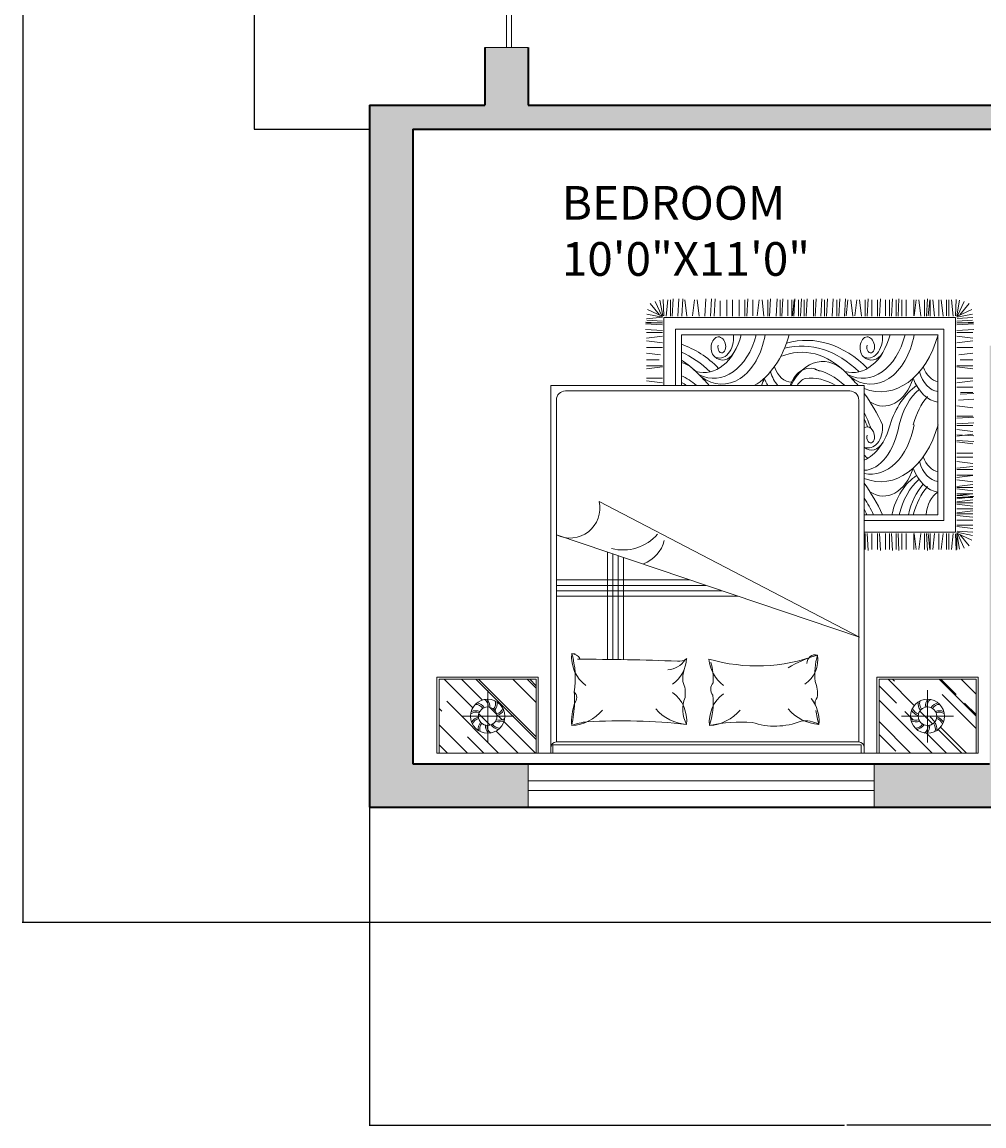
# Model space of a CAD drawing. Units: inches. Extents: x 2540 to 3167, y 3083 to 4007.
# Tile 1 of 15: x 2540 to 2740, y 3083 to 3313. Entities that reach past the tile are written whole.
import ezdxf

# ---------------------------------------------------------------- set-up
doc = ezdxf.new("R2010")
doc.units = ezdxf.units.IN
for name, color, linetype, lineweight in [('A-ANNO-DIMS', 2, 'Continuous', 18), ('A-AREA-IDEN', 7, 'Continuous', 18), ('A-DOOR', 4, 'Continuous', 18), ('A-FLOR-EDGE', 7, 'Continuous', 25), ('A-FURN', 8, 'Continuous', 13), ('A-GLAZ', 4, 'Continuous', 18)]:
    doc.layers.add(name, color=color, linetype=linetype, lineweight=lineweight)
doc.layers.add('A-WALL', color=143, linetype='Continuous', lineweight=35, true_color=0x7aafdf)
doc.layers.add('A-WALL-PATT', color=143, linetype='Continuous', lineweight=13, true_color=0x7aafdf)
doc.styles.get("Standard").update_dxf_attribs({"font": 'arial.ttf'})
doc.dimstyles.get("Standard").update_dxf_attribs({"dimtxt": 0.18, "dimasz": 0.18, "dimexe": 0.18, "dimexo": 0.0625, "dimgap": 0.09, "dimtad": 0, "dimtih": 1, "dimtoh": 1, "dimdec": 4, "dimzin": 0, "dimdsep": 46, "dimtxsty": 'Standard', "dimcen": 0.09, "dimadec": 0, "dimazin": 0, "dimtfac": 1, "dimtdec": 4, "dimtofl": 0, "dimtmove": 0, "dimatfit": 3, "dimfxl": 1, "dimtolj": 1, "dimtzin": 0, "dimarcsym": 0})

# ---------------------------------------------------------------- blocks, each defined once
blk = doc.blocks.new('A$C64B41DC1')
for p, q in [((0, 2.5079), (2.9903, 2.5079)), ((0, 2.0879), (0, 2.5079)), ((0.012, 2.4618), (0.0581, 2.5079)), ((0.012, 2.3515), (0.1684, 2.5079)), ((0.012, 2.0999), (0.012, 2.5079)), ((0.0543, 2.2213), (0.3409, 2.5079)), ((0.1689, 2.4179), (0.2589, 2.5079)), ((0.3265, 2.386), (0.4484, 2.5079)), ((0.3699, 2.3332), (0.5445, 2.5079)), ((0.548, 2.5079), (0.548, 2.0999)), ((0.56, 2.5079), (0.56, 2.0879)), ((0.6301, 2.5079), (0.6301, 0.4779)), ((0.6401, 2.461), (0.6401, 2.5079)), ((0.6401, 2.5079), (2.344, 2.5079)), ((2.344, 2.5079), (2.3601, 2.5079)), ((2.344, 2.5079), (2.344, 2.461)), ((2.3601, 2.5079), (2.3601, 2.4761)), ((2.3601, 0.4779), (2.3601, 2.5079)), ((2.4303, 2.5079), (2.4303, 2.0879)), ((2.4423, 2.5079), (2.4423, 2.0999)), ((2.4423, 2.3333), (2.6169, 2.5079)), ((2.4423, 2.2145), (2.7357, 2.5079)), ((2.705, 2.398), (2.8149, 2.5079)), ((2.7691, 2.3772), (2.8998, 2.5079)), ((2.7819, 2.3646), (2.9252, 2.5079)), ((2.9783, 2.0999), (2.9783, 2.5079)), ((2.9903, 2.0879), (2.9903, 2.5079)), ((0.2804, 2.1597), (0.2804, 2.4481)), ((2.344, 2.461), (0.6401, 2.461)), ((0.6601, 2.4461), (1.4951, 2.4461)), ((0.6601, 2.4461), (0.6601, 0.5579)), ((1.4951, 2.4461), (0.6697, 2.4461)), ((2.3301, 2.4461), (1.4951, 2.4461)), ((2.3301, 0.5579), (2.3301, 2.4461)), ((2.4423, 2.404), (2.5354, 2.4971)), ((2.7099, 2.1597), (2.7099, 2.4481)), ((0.2157, 2.0999), (0.548, 2.4322)), ((0.2299, 2.0999), (0.548, 2.418)), ((0.2311, 2.2906), (0.2937, 2.3532)), ((0.3405, 2.3039), (0.3605, 2.3238)), ((2.6158, 2.3088), (2.6313, 2.3243)), ((2.6674, 2.2756), (2.7382, 2.3464)), ((2.7249, 2.3076), (2.7512, 2.3339)), ((2.7914, 2.1846), (2.9783, 2.3715)), ((0.012, 2.261), (0.0275, 2.2765)), ((0.0404, 2.0999), (0.1982, 2.2578)), ((0.1362, 2.3039), (0.4246, 2.3039)), ((0.2905, 2.2539), (0.3304, 2.2938)), ((2.8541, 2.3039), (2.5657, 2.3039)), ((2.5849, 2.2779), (2.6158, 2.3088)), ((2.7746, 2.0999), (2.9783, 2.3036)), ((2.9144, 2.2312), (2.9783, 2.2951)), ((0.1365, 2.0999), (0.251, 2.2144)), ((0.4194, 2.0999), (0.548, 2.2285)), ((2.4423, 2.1353), (2.5382, 2.2312)), ((2.4918, 2.0999), (2.6366, 2.2447)), ((0.4986, 2.0999), (0.548, 2.1493)), ((0.5127, 2.0999), (0.548, 2.1352)), ((2.7831, 2.0999), (2.8678, 2.1846)), ((2.8962, 2.0999), (2.9783, 2.182)), ((0.56, 2.0879), (0, 2.0879)), ((0.548, 2.0999), (0.012, 2.0999)), ((2.4303, 2.0879), (2.9903, 2.0879)), ((2.4423, 2.0999), (2.9783, 2.0999)), ((2.5172, 2.0999), (2.5269, 2.1096)), ((0.9415, 1.9902), (0.9415, 1.3975)), ((0.9715, 1.9906), (0.9715, 1.4076)), ((1.0015, 1.991), (1.0015, 1.4177)), ((1.0315, 1.9916), (1.0315, 1.4279)), ((2.3349, 1.8678), (0.6613, 1.3029)), ((0.8956, 1.1191), (2.3349, 1.8678)), ((1.6636, 1.6412), (0.6601, 1.6412)), ((1.5748, 1.6112), (0.6601, 1.6112)), ((2.3665, 1.295), (2.3665, 1.3839)), ((2.377, 1.295), (2.3822, 1.3891)), ((2.4032, 1.295), (2.4032, 1.3839)), ((2.4346, 1.295), (2.4346, 1.3839)), ((2.4451, 1.295), (2.4503, 1.3891)), ((2.4774, 1.2957), (2.4774, 1.3837)), ((2.5, 1.295), (2.5, 1.3839)), ((2.5105, 1.295), (2.5157, 1.3891)), ((2.5367, 1.295), (2.5367, 1.3839)), ((2.5471, 1.295), (2.5524, 1.3891)), ((2.5681, 1.295), (2.5681, 1.3839)), ((2.5918, 1.295), (2.5918, 1.3839)), ((2.6346, 1.2957), (2.6346, 1.3837)), ((2.6362, 1.2957), (2.6467, 1.3839)), ((2.6729, 1.295), (2.6624, 1.3839)), ((2.6938, 1.295), (2.6938, 1.3839)), ((2.7043, 1.295), (2.7095, 1.3891)), ((2.7127, 1.2957), (2.7232, 1.3839)), ((2.7253, 1.295), (2.7253, 1.3839)), ((2.7494, 1.295), (2.7389, 1.3839)), ((2.7718, 1.295), (2.7718, 1.3839)), ((2.7959, 1.295), (2.7854, 1.3839)), ((2.8146, 1.2957), (2.8146, 1.3837)), ((2.8146, 1.2957), (2.8146, 1.3837)), ((2.8282, 1.295), (2.8282, 1.3839)), ((2.8282, 1.295), (2.8282, 1.3839)), ((2.8523, 1.295), (2.8418, 1.3839)), ((2.8523, 1.295), (2.8418, 1.3839)), ((2.8653, 1.2966), (2.8688, 1.3861)), ((2.8711, 1.2957), (2.8711, 1.3837)), ((2.8711, 1.2957), (2.8875, 1.3822)), ((2.8765, 1.2958), (2.9132, 1.3758)), ((2.8893, 1.3011), (2.9394, 1.3636)), ((2.3601, 1.2873), (2.8639, 1.2873)), ((2.8639, 1.2873), (2.8639, 0.1018)), ((2.8713, 1.2927), (2.954, 1.3315)), ((2.8717, 1.2884), (2.9588, 1.3058)), ((2.8744, 1.2817), (2.9603, 1.2869)), ((2.3601, 1.2233), (2.7999, 1.2233)), ((2.7999, 1.2233), (2.7999, 0.1658)), ((2.8716, 1.2565), (2.9605, 1.2669)), ((2.8716, 1.2212), (2.9605, 1.2212)), ((2.8723, 1.2489), (2.9603, 1.2489)), ((2.3601, 1.1913), (2.7679, 1.1912)), ((2.7679, 1.1912), (2.7679, 0.1978)), ((2.8716, 1.1947), (2.9605, 1.2052)), ((2.8716, 1.181), (2.9605, 1.1705)), ((2.8716, 1.1595), (2.9605, 1.1595)), ((2.8723, 1.1872), (2.9603, 1.1872)), ((2.8716, 1.133), (2.9605, 1.1435)), ((2.8716, 1.1193), (2.9605, 1.1088)), ((2.8716, 1.1035), (2.9605, 1.093)), ((2.8723, 1.1255), (2.9603, 1.1255)), ((2.8716, 1.0965), (2.9605, 1.0965)), ((2.8716, 1.086), (2.9657, 1.0913)), ((2.8716, 1.0756), (2.9605, 1.0756)), ((2.8716, 1.0491), (2.9605, 1.0596)), ((2.8723, 1.0858), (2.9605, 1.0753)), ((2.8723, 1.0416), (2.9603, 1.0416)), ((2.8716, 1.0354), (2.9605, 1.0249)), ((2.8723, 0.9987), (2.9605, 1.0092)), ((2.8723, 0.985), (2.9605, 0.9745)), ((2.8716, 0.9346), (2.9605, 0.9241)), ((2.8723, 0.9735), (2.9603, 0.9735)), ((2.8723, 0.9408), (2.9603, 0.9408)), ((2.8723, 0.8979), (2.9605, 0.9084)), ((2.8723, 0.8726), (2.9603, 0.8726)), ((2.8716, 0.7885), (2.9605, 0.799)), ((2.8723, 0.8505), (2.9603, 0.8505)), ((2.8716, 0.7818), (2.9657, 0.787)), ((2.8716, 0.7503), (2.9657, 0.7556)), ((2.8723, 0.7571), (2.9605, 0.7466)), ((2.8716, 0.7204), (2.9605, 0.7309)), ((2.8716, 0.6995), (2.9605, 0.6995)), ((2.8716, 0.689), (2.9657, 0.6838)), ((2.8716, 0.6576), (2.9657, 0.6523)), ((2.8716, 0.6471), (2.9605, 0.6471)), ((2.8716, 0.5903), (2.9605, 0.6007)), ((2.882, 0.5582), (2.9657, 0.5536)), ((0.7101, 0.5079), (2.2801, 0.5079)), ((2.8716, 0.4877), (2.9603, 0.4877)), ((2.8909, 0.5263), (2.9657, 0.5222)), ((2.8928, 0.5169), (2.9605, 0.5169)), ((0.6301, 0.4779), (2.3601, 0.4779)), ((1.2465, 0.4625), (1.1576, 0.452)), ((1.2465, 0.4365), (1.1577, 0.4365)), ((1.2542, 0.1018), (1.2542, 0.4779)), ((1.3182, 0.1658), (1.3182, 0.4779)), ((1.3502, 0.1978), (1.3502, 0.4779)), ((2.8716, 0.4625), (2.9605, 0.452)), ((2.8716, 0.4365), (2.9603, 0.4365)), ((1.2465, 0.3746), (1.1576, 0.3851)), ((1.2465, 0.3684), (1.1577, 0.3684)), ((2.8716, 0.3746), (2.9605, 0.3851)), ((2.8716, 0.3684), (2.9603, 0.3684)), ((1.2355, 0.3092), (1.1576, 0.3)), ((1.2285, 0.3357), (1.1577, 0.3357)), ((2.8826, 0.3092), (2.9605, 0.3)), ((2.8896, 0.3357), (2.9603, 0.3357)), ((1.2457, 0.2676), (1.1577, 0.2676)), ((2.8723, 0.2676), (2.9603, 0.2676)), ((1.2457, 0.2423), (1.1576, 0.2319)), ((1.2465, 0.2057), (1.1576, 0.2161)), ((1.2465, 0.1847), (1.1576, 0.1847)), ((2.7679, 0.1978), (1.3502, 0.1978)), ((2.8716, 0.2057), (2.9605, 0.2161)), ((2.8716, 0.1847), (2.9605, 0.1847)), ((2.8723, 0.2423), (2.9605, 0.2319)), ((1.2465, 0.1742), (1.1524, 0.169)), ((1.2465, 0.1428), (1.1524, 0.1376)), ((1.2465, 0.1334), (1.1524, 0.1281)), ((1.2465, 0.1323), (1.1576, 0.1323)), ((1.2465, 0.1323), (1.1576, 0.1323)), ((1.2465, 0.1229), (1.1588, 0.1168)), ((2.7999, 0.1658), (1.3182, 0.1658)), ((2.8716, 0.1742), (2.9657, 0.169)), ((2.8716, 0.1428), (2.9657, 0.1376)), ((2.8716, 0.1334), (2.9657, 0.1281)), ((2.8716, 0.1323), (2.9605, 0.1323)), ((2.8716, 0.1229), (2.9593, 0.1168)), ((1.2465, 0.1), (1.1576, 0.1105)), ((1.2464, 0.1007), (1.1592, 0.0833)), ((1.2468, 0.0964), (1.1641, 0.0576)), ((1.2288, 0.088), (1.1787, 0.0255)), ((1.2415, 0.0933), (1.2049, 0.0133)), ((1.247, 0.0934), (1.2306, 0.0069)), ((1.2527, 0.0925), (1.2493, 0.003)), ((2.8639, 0.1018), (1.2542, 0.1018)), ((1.2658, 0.0941), (1.2762, 0.0052)), ((1.2899, 0.0941), (1.2899, 0.0052)), ((1.2999, 0.0941), (1.3051, 0)), ((1.3313, 0.0941), (1.3365, 0)), ((1.3523, 0.0941), (1.3575, 0)), ((1.3804, 0.0941), (1.3699, 0.0052)), ((1.4119, 0.0934), (1.4223, 0.0052)), ((1.4485, 0.0941), (1.438, 0.0052)), ((1.48, 0.0941), (1.4852, 0)), ((1.5114, 0.0941), (1.5166, 0)), ((1.5323, 0.0941), (1.5376, 0)), ((1.5638, 0.0941), (1.5638, 0.0105)), ((1.6021, 0.0941), (1.6021, 0.0052)), ((1.6336, 0.0941), (1.6336, 0.0052)), ((1.6702, 0.0941), (1.6702, 0.0052)), ((1.7017, 0.0941), (1.7017, 0.0052)), ((1.7122, 0.0941), (1.7174, 0)), ((1.7445, 0.0934), (1.7445, 0.0054)), ((1.7698, 0.0934), (1.7803, 0.0052)), ((1.8065, 0.0941), (1.796, 0.0052)), ((1.8274, 0.0941), (1.8274, 0.0052)), ((1.8379, 0.0941), (1.8431, 0)), ((1.8746, 0.0941), (1.8798, 0)), ((1.8955, 0.0941), (1.8955, 0.0052)), ((1.906, 0.0941), (1.9113, 0)), ((1.9384, 0.0934), (1.9384, 0.0054)), ((1.9609, 0.0941), (1.9609, 0.0052)), ((1.9636, 0.0934), (1.9741, 0.0052)), ((1.9714, 0.0941), (1.9766, 0)), ((1.9976, 0.0941), (1.9976, 0.0052)), ((2.0081, 0.0941), (2.0133, 0)), ((2.029, 0.0941), (2.029, 0.0052)), ((2.0395, 0.0941), (2.0447, 0)), ((2.0797, 0.0941), (2.0797, 0.0052)), ((2.0902, 0.0941), (2.0954, 0)), ((2.1216, 0.0941), (2.1269, 0)), ((2.1412, 0.0941), (2.1412, 0.0052)), ((2.1517, 0.0941), (2.1569, 0)), ((2.1831, 0.0941), (2.1884, 0)), ((2.2093, 0.0941), (2.2093, 0.0052)), ((2.2198, 0.0941), (2.225, 0)), ((2.2512, 0.0941), (2.2565, 0)), ((2.2603, 0.0934), (2.2707, 0.0052)), ((2.2969, 0.0941), (2.2864, 0.0052)), ((2.3089, 0.0934), (2.3193, 0.0052)), ((2.3455, 0.0941), (2.3351, 0.0052)), ((2.3665, 0.0941), (2.3665, 0.0052)), ((2.377, 0.0941), (2.3822, 0)), ((2.4032, 0.0941), (2.4032, 0.0052)), ((2.4346, 0.0941), (2.4346, 0.0052)), ((2.4451, 0.0941), (2.4503, 0)), ((2.4774, 0.0934), (2.4774, 0.0054)), ((2.5, 0.0941), (2.5, 0.0052)), ((2.5105, 0.0941), (2.5157, 0)), ((2.5367, 0.0941), (2.5367, 0.0052)), ((2.5471, 0.0941), (2.5524, 0)), ((2.5681, 0.0941), (2.5681, 0.0052)), ((2.5918, 0.0941), (2.5918, 0.0052)), ((2.6346, 0.0934), (2.6346, 0.0054)), ((2.6362, 0.0934), (2.6467, 0.0052)), ((2.6729, 0.0941), (2.6624, 0.0052)), ((2.6938, 0.0941), (2.6938, 0.0052)), ((2.7043, 0.0941), (2.7095, 0)), ((2.7127, 0.0934), (2.7232, 0.0052)), ((2.7253, 0.0941), (2.7253, 0.0052)), ((2.7494, 0.0941), (2.7389, 0.0052)), ((2.7718, 0.0941), (2.7718, 0.0052)), ((2.7959, 0.0941), (2.7854, 0.0052)), ((2.8146, 0.0934), (2.8146, 0.0054)), ((2.8282, 0.0941), (2.8282, 0.0052)), ((2.8523, 0.0941), (2.8418, 0.0052)), ((2.8653, 0.0925), (2.8688, 0.003)), ((2.8711, 0.0934), (2.8875, 0.0069)), ((2.8713, 0.0964), (2.954, 0.0576)), ((2.8717, 0.1007), (2.9588, 0.0833)), ((2.8744, 0.1074), (2.9603, 0.1022)), ((2.8765, 0.0933), (2.9132, 0.0133)), ((2.8893, 0.088), (2.9394, 0.0255))]:
    blk.add_line(p, q)
at = {"ltscale": 10}
for p, q in [((1.4859, 1.5812), (0.6601, 1.5812)), ((1.397, 1.5512), (0.6601, 1.5512))]:
    blk.add_line(p, q, dxfattribs=at)
for centre, radius in [((0.2804, 2.3039), 0.0942), ((2.7099, 2.3039), 0.0942), ((0.2804, 2.3039), 0.051), ((2.7099, 2.3039), 0.051)]:
    blk.add_circle(centre, radius)
for centre, radius, start, end in [((0.6601, 2.4761), 0.03, 180, 270), ((2.3301, 2.4761), 0.03, 270, 0), ((0.2887, 2.3745), 0.0605, 172.17003, 218.48975), ((0.2828, 2.3731), 0.0462, 160.30017, 220.53802), ((0.3286, 2.3561), 0.0605, 136.17003, 182.48975), ((0.3231, 2.3585), 0.0462, 124.30017, 184.53802), ((0.3501, 2.3178), 0.0605, 100.17003, 146.48975), ((2.6402, 2.3178), 0.0605, 33.51025, 79.82997), ((2.6672, 2.3585), 0.0462, 355.46198, 55.69983), ((2.6617, 2.3561), 0.0605, 357.51025, 43.82997), ((2.7075, 2.3731), 0.0462, 319.46198, 19.69983), ((2.7016, 2.3745), 0.0605, 321.51025, 7.82997), ((0.2457, 2.3659), 0.0605, 208.17003, 254.48975), ((0.2417, 2.3614), 0.0462, 196.30017, 256.53802), ((0.347, 2.323), 0.0462, 88.30017, 148.53802), ((0.3449, 2.2742), 0.0605, 64.17003, 110.48975), ((0.3455, 2.2802), 0.0462, 52.30017, 112.53802), ((1.0526, 2.3302), 0.3085, 175.30484, 198.69419), ((-0.8702, 2.0941), 1.6364, 4.80985, 9.18918), ((0.8579, 2.6278), 0.2948, 247.51785, 264.26696), ((0.728, 2.111), 0.245, 40.4189, 85.9871), ((1.0164, 5.7096), 3.3803, 266.81337, 276.16021), ((1.3963, 2.1044), 0.245, 94.0129, 139.5811), ((1.1858, 2.3288), 0.1943, 306.5711, 5.88998), ((1.5348, 2.2652), 0.1767, 151.77364, 201.69827), ((1.6986, 2.3355), 0.1943, 174.11002, 233.4289), ((1.1481, 2.2311), 0.3783, 353.49469, 19.18669), ((1.6871, 3.192), 0.8561, 257.74383, 273.62843), ((1.4882, 2.111), 0.245, 40.4189, 85.9871), ((1.8674, 1.9709), 0.3878, 68.20259, 108.9817), ((2.1269, 2.1044), 0.245, 94.0129, 139.5811), ((2.0342, 2.4856), 0.1563, 261.59582, 298.90918), ((1.9165, 2.3288), 0.1943, 333.73715, 5.88998), ((2.6058, 2.2028), 0.517, 163.60457, 172.3273), ((2.6448, 2.2802), 0.0462, 67.46198, 127.69983), ((2.6454, 2.2742), 0.0605, 69.51025, 115.82997), ((2.6433, 2.323), 0.0462, 31.46198, 91.69983), ((2.7486, 2.3614), 0.0462, 283.46198, 343.69983), ((2.7446, 2.3659), 0.0605, 285.51025, 331.82997), ((0.2153, 2.3276), 0.0462, 232.30017, 292.53802), ((0.2158, 2.3336), 0.0605, 244.17003, 290.48975), ((0.2138, 2.2848), 0.0462, 268.30017, 328.53802), ((0.2107, 2.29), 0.0605, 280.17003, 326.48975), ((0.2779, 2.2347), 0.0462, 340.30017, 40.53802), ((0.272, 2.2333), 0.0605, 352.17003, 38.48975), ((0.3191, 2.2464), 0.0462, 16.30017, 76.53802), ((0.3151, 2.2419), 0.0605, 28.17003, 74.48975), ((2.6752, 2.2419), 0.0605, 105.51025, 151.82997), ((2.6712, 2.2464), 0.0462, 103.46198, 163.69983), ((2.7182, 2.2333), 0.0605, 141.51025, 187.82997), ((2.7123, 2.2347), 0.0462, 139.46198, 199.69983), ((2.7796, 2.29), 0.0605, 213.51025, 259.82997), ((2.7765, 2.2848), 0.0462, 211.46198, 271.69983), ((2.7744, 2.3336), 0.0605, 249.51025, 295.82997), ((2.775, 2.3276), 0.0462, 247.46198, 307.69983), ((0.2377, 2.2493), 0.0462, 304.30017, 4.53802), ((0.2322, 2.2517), 0.0605, 316.17003, 2.48975), ((0.7274, 2.2013), 0.0446, 314.4736, 42.17134), ((-1.6008, 2.277), 2.3618, 357.39054, 358.88764), ((1.204, 2.1778), 0.1681, 337.01697, 7.53676), ((1.9165, 2.3288), 0.1943, 320.94042, 333.73715), ((2.1347, 2.2313), 0.0459, 165.35061, 223.26844), ((1.9346, 2.1778), 0.1681, 337.01697, 7.53676), ((2.7581, 2.2517), 0.0605, 177.51025, 223.82997), ((2.7526, 2.2493), 0.0462, 175.46198, 235.69983), ((0.9385, 1.978), 0.1943, 126.5711, 185.88998), ((0.2688, 2.0945), 0.4956, 344.0243, 8.70709), ((1.7059, 1.9714), 0.204, 127.11975, 175.09005), ((1.5671, 2.1546), 0.0547, 142.08329, 220.902), ((1.1858, 1.9714), 0.1943, 4.31813, 53.4289), ((1.5415, 2.0969), 0.1834, 175.22328, 196.23004), ((1.1965, 2.0983), 0.3299, 343.79543, 3.55541), ((1.9394, 1.991), 0.1651, 351.26213, 55.75721), ((2.4617, 2.0719), 0.3745, 173.82958, 196.4356), ((1.2687, 1.9248), 0.1223, 33.62799, 86.47438), ((1.7676, 1.0629), 0.9631, 69.65065, 105.96307), ((2.2748, 2.5795), 0.6373, 238.34989, 254.31375), ((2.0911, 2.0123), 0.0478, 179.77267, 283.80184), ((0.7417, 2.0149), 0.057, 273.47085, 328.54118), ((0.728, 2.2025), 0.245, 274.0129, 278.34166), ((0.7246, 18.8439), 16.8552, 270.17399, 272.05214), ((1.3401, 1.9404), 0.0603, 49.09906, 101.37023), ((1.0747, 1.2871), 0.1871, 14.1863, 69.12121), ((1.0274, 1.1334), 0.2527, 40.62904, 104.37123), ((0.7347, 1.1553), 0.1649, 347.31088, 116.44537), ((0.7101, 0.5579), 0.05, 180, 270), ((2.2801, 0.5579), 0.05, 270, 0)]:
    blk.add_arc(centre, radius, start, end)
for centre, major_axis, ratio, start_param, end_param in [((1.9938, 1.6262), (0, -0.7531), 0.68, 0.797284, 0.954936), ((2.0643, 1.466), (0, -0.5322), 0.68, 7.239912, 7.311536), ((1.9052, 1.7397), (0, -0.9842), 0.68, 0.74745, 0.979724), ((2.7455, 1.3081), (0, 0.3614), 0.68, 1.900046, 2.742661), ((2.7868, 1.3081), (0, 0.3614), 0.68, 1.900046, 2.614747), ((2.8372, 1.3081), (0, 0.3614), 0.68, 1.900046, 2.479658), ((2.8607, 1.3211), (0, 0.3614), 0.68, 1.938265, 2.479658), ((2.8057, 1.2079), (0, -0.1524), 0.68, 4.821745, 5.895886), ((2.4665, 0.8216), (0, -0.2664), 0.68, 2.006169, 3.565187), ((2.4513, 0.5069), (0, 0.502), 0.68, 5.095327, 6.553458), ((2.7862, 0.8069), (0, -0.2615), 0.68, 3.244645, 4.205018), ((2.396, 0.6032), (0, 0.3641), 0.68, -1.3172, 0.145284), ((2.7784, 0.8289), (0, -0.1802), 0.68, 3.227058, 4.318474), ((2.3507, 0.5642), (0.0073, 0.3819), 0.56205, -1.21172, -0.009991), ((2.7821, 0.7971), (0, -0.1589), 0.68, 3.272942, 4.229533), ((2.2964, 0.5771), (0, -0.3263), 0.68, 1.938944, 2.850232), ((2.0403, 1.6015), (0, -0.8763), 0.68, 6.849801, 6.887077), ((2.4005, 0.7132), (0, -0.1214), 0.68, 2.284368, 3.652258), ((2.3834, 0.7081), (0, 0.1147), 0.68, 4.593909, 6.585576), ((2.3961, 0.7628), (0, -0.0317), 0.68, 1.462497, 5.046281), ((2.3774, 0.7653), (0, -0.0593), 0.68, 5.841311, 7.755362), ((1.9938, 1.1295), (-0.0678, 0.7439), 0.610498, 3.917146, 4.063997), ((2.0643, 0.9693), (0, -0.5322), 0.68, 7.239912, 7.336618), ((1.9052, 1.243), (0, -0.9842), 0.68, 0.74745, 0.979724), ((2.7455, 0.8114), (-0.0599, 0.3735), 0.695517, 1.775813, 2.548612), ((2.7868, 0.8114), (0, 0.3614), 0.68, 1.900046, 2.614747), ((2.8607, 0.8243), (0, 0.3614), 0.68, 1.938265, 2.479658), ((2.4665, 0.3249), (0, -0.2664), 0.68, 2.006169, 3.565187), ((2.4513, 0.0102), (0, 0.502), 0.68, 5.095327, 6.553458), ((2.7862, 0.3102), (0, -0.2615), 0.68, 3.244645, 4.205018), ((2.7784, 0.3322), (0, -0.1802), 0.68, 3.227058, 4.318474), ((1.242, 0.9693), (0, -0.5322), 0.68, 6.586764, 6.677612), ((1.1714, 1.1295), (-0.1157, 0.7241), 0.59432, 3.291697, 3.50733), ((1.474, 0.0804), (0, -0.3263), 0.68, 1.938944, 3.339184), ((1.0828, 1.243), (0, -0.9842), 0.68, 0.565948, 0.680366), ((1.5283, 0.0674), (0, -0.3703), 0.68, 1.930561, 3.464283), ((1.5736, 0.1065), (0, 0.3641), 0.68, -1.3172, 0.476403), ((1.6289, 0.0102), (0, 0.502), 0.68, 6.655152, 6.661293), ((1.6289, 0.0102), (0, 0.502), 0.68, 5.095327, 5.911219), ((1.6442, 0.3249), (0, -0.2664), 0.68, 2.006169, 2.182797), ((1.9638, 0.3102), (0, -0.2615), 0.68, 4.015924, 4.205018), ((1.956, 0.3322), (0, -0.1802), 0.68, 3.770744, 4.318474), ((1.9597, 0.3004), (0, -0.1589), 0.68, 3.14258, 4.229533), ((2.0606, 0.5616), (0, -0.1803), 0.68, 5.194792, 5.929328), ((2.0606, 0.5616), (0, -0.1803), 0.68, 5.194792, 6.723255), ((2.1315, 0.6603), (0, -0.3155), 0.68, 5.328638, 6.949396), ((2.0549, 0.5656), (0, -0.1303), 0.68, 5.450951, 6.054641), ((2.0643, 0.9693), (0, -0.5322), 0.68, 6.20013, 6.677612), ((1.9938, 1.1295), (-0.0678, 0.7439), 0.610498, 3.199135, 3.592282), ((2.2964, 0.0804), (0, -0.3263), 0.68, 1.938944, 3.339184), ((1.9052, 1.243), (0, -0.9842), 0.68, 0.565948, 0.680366), ((2.3507, 0.0674), (0, -0.3703), 0.68, 1.930561, 3.464283), ((2.396, 0.1065), (0, 0.3641), 0.68, -1.3172, 0.476403), ((2.4513, 0.0102), (0, 0.502), 0.68, 6.655152, 6.661293), ((2.7821, 0.3004), (0, -0.1589), 0.68, 3.272942, 4.229533), ((1.1933, 0.9181), (0, -0.624), 0.68, 0.378672, 0.625379), ((1.3091, 0.6603), (0, -0.3155), 0.68, 6.475719, 6.949396), ((1.1911, 1.1066), (0, 0.8458), 0.68, 3.421828, 3.728616), ((1.2179, 1.1047), (0, -0.8763), 0.68, 6.507006, 6.887077), ((2.0157, 0.9181), (0, -0.624), 0.68, -0.280078, 0.625379), ((2.0135, 1.1066), (0, 0.8458), 0.68, 2.978727, 3.728616), ((2.0403, 1.1047), (0, -0.8763), 0.68, 6.099302, 6.887077), ((1.555, 0.2685), (0, -0.0593), 0.68, 3.732151, 7.755362), ((1.5781, 0.2165), (0, -0.1214), 0.68, 2.284368, 3.726131), ((1.561, 0.2114), (0, 0.1147), 0.68, 4.593909, 6.647252), ((2.3774, 0.2685), (0, -0.0593), 0.68, 3.732151, 7.755362), ((2.4005, 0.2165), (0, -0.1214), 0.68, 2.284368, 3.726131), ((2.3834, 0.2114), (0, 0.1147), 0.68, 4.593909, 6.647252), ((1.5737, 0.2661), (0, -0.0317), 0.68, 1.462497, 5.046281), ((2.3961, 0.2661), (0, -0.0317), 0.68, 1.462497, 5.046281)]:
    blk.add_ellipse(centre, major_axis=major_axis, ratio=ratio, start_param=start_param, end_param=end_param)
blk = doc.blocks.new('DOOR-SLIDING-96IN')
for p, q in [((9, 96), (0, 96)), ((3.5, 48), (3.5, 96)), ((4.5, 0), (4.5, 96)), ((5.5, 48), (3.5, 48)), ((5.5, 0), (5.5, 48)), ((9, 0), (0, 0))]:
    blk.add_line(p, q)
blk = doc.blocks.new('WIN-72IN')
for p, q in [((9, 72), (0, 72)), ((3.5, 0), (3.5, 72)), ((5.5, 0), (5.5, 72)), ((9, 0), (0, 0))]:
    blk.add_line(p, q)
blk = doc.blocks.new('*D44')
at = {"layer": 'A-ANNO-DIMS', "color": 0, "lineweight": -2, "transparency": 16777216}
for p, q in [((2771.45, 3964.71), (2540.23, 3964.71)), ((2540.41, 3964.53), (2540.41, 3545.4)), ((2540.41, 3125.89), (2540.41, 3545.03)), ((2810.45, 3125.71), (2540.23, 3125.71))]:
    blk.add_line(p, q, dxfattribs=at)
at = {"layer": 'A-ANNO-DIMS', "color": 0, "transparency": 16777216}
for points in [[(2540.38, 3964.53), (2540.44, 3964.53), (2540.41, 3964.71)], [(2540.38, 3125.89), (2540.44, 3125.89), (2540.41, 3125.71)]]:
    blk.add_solid(points, dxfattribs=at)
at = {"layer": 'Defpoints', "color": 0, "transparency": 16777216}
for p in [(2540.41, 3964.71), (2771.51, 3964.71), (2810.51, 3125.71)]:
    blk.add_point(p, dxfattribs=at)
at = {"layer": 'A-ANNO-DIMS', "color": 0, "transparency": 16777216, "insert": (2540.41, 3545.21), "char_height": 0.18, "attachment_point": 5}
blk.add_mtext('\\A1;839', dxfattribs=at)
blk = doc.blocks.new('*D45')
at = {"layer": 'A-ANNO-DIMS', "color": 0, "lineweight": -2, "transparency": 16777216}
for p, q in [((2612.51, 3149.65), (2612.51, 3083.43)), ((2810.51, 3125.65), (2810.51, 3083.43)), ((2612.69, 3083.61), (2711.23, 3083.61)), ((2810.33, 3083.61), (2711.79, 3083.61))]:
    blk.add_line(p, q, dxfattribs=at)
at = {"layer": 'A-ANNO-DIMS', "color": 0, "transparency": 16777216}
for points in [[(2612.69, 3083.64), (2612.69, 3083.58), (2612.51, 3083.61)], [(2810.33, 3083.64), (2810.33, 3083.58), (2810.51, 3083.61)]]:
    blk.add_solid(points, dxfattribs=at)
at = {"layer": 'Defpoints', "color": 0, "transparency": 16777216}
for p in [(2612.51, 3149.71), (2810.51, 3125.71), (2810.51, 3083.61)]:
    blk.add_point(p, dxfattribs=at)
at = {"layer": 'A-ANNO-DIMS', "color": 0, "transparency": 16777216, "insert": (2711.51, 3083.61), "char_height": 0.18, "attachment_point": 5}
blk.add_mtext('\\A1;198', dxfattribs=at)

msp = doc.modelspace()

# ---------------------------------------------------------------- hatches: boundary and pattern name
at = {"layer": 'A-WALL-PATT'}
h = msp.add_hatch(color=256, dxfattribs=at)
h.dxf.hatch_style = 1
h.paths.add_polyline_path([(2805.51, 3803.71), (2800.51, 3803.71), (2800.51, 3799.71), (2621.51, 3799.71), (2621.51, 3823.71), (2612.51, 3823.71), (2612.51, 3794.71), (2636.51, 3794.71), (2636.51, 3782.71), (2645.51, 3782.71), (2645.51, 3794.71), (2805.51, 3794.71)])
h.paths.add_polyline_path([(2810.51, 3564.71), (2868.51, 3564.71), (2868.51, 3627.71), (2872.51, 3627.71), (2872.51, 3636.71), (2864.51, 3636.71), (2864.51, 3674.71), (2797.51, 3674.71), (2797.51, 3669.71), (2801.51, 3669.71), (2801.51, 3628.63), (2806.51, 3628.63), (2806.51, 3669.71), (2859.51, 3669.71), (2859.51, 3573.71), (2806.51, 3573.71), (2806.51, 3598.63), (2801.51, 3598.63), (2801.51, 3549.71), (2645.51, 3549.71), (2645.51, 3573.71), (2636.51, 3573.71), (2636.51, 3516.71), (2645.51, 3516.71), (2645.51, 3540.71), (2801.51, 3540.71), (2801.51, 3504.71), (2801.51, 3500.71), (2806.51, 3500.71), (2806.51, 3504.71), (2859.51, 3504.71), (2859.51, 3420.71), (2806.51, 3420.71), (2806.51, 3470.71), (2801.51, 3470.71), (2801.51, 3420.71), (2797.51, 3420.71), (2797.51, 3415.71), (2864.51, 3415.71), (2864.51, 3453.71), (2868.51, 3453.71), (2868.51, 3513.71), (2810.51, 3513.71)])
h.paths.add_polyline_path([(2645.51, 3415.71), (2761.51, 3415.71), (2761.51, 3420.71), (2645.51, 3420.71), (2645.51, 3444.71), (2636.51, 3444.71), (2636.51, 3403.71), (2645.51, 3403.71)])
h.paths.add_polyline_path([(2645.51, 3307.71), (2636.51, 3307.71), (2636.51, 3295.71), (2612.51, 3295.71), (2612.51, 3149.71), (2645.51, 3149.71), (2645.51, 3158.71), (2621.51, 3158.71), (2621.51, 3290.71), (2801.51, 3290.71), (2801.51, 3286.71), (2806.51, 3286.71), (2806.51, 3295.71), (2645.51, 3295.71)])
h.paths.add_polyline_path([(2762.01, 3158.71), (2746.51, 3158.71), (2746.51, 3240.71), (2750.51, 3240.71), (2750.51, 3245.71), (2741.51, 3245.71), (2741.51, 3158.71), (2717.51, 3158.71), (2717.51, 3149.71), (2762.01, 3149.71)], flags=17)
h.paths.add_polyline_path([(2810.51, 3173.71), (2822.51, 3173.71), (2822.51, 3182.71), (2806.51, 3182.71), (2806.51, 3250.71), (2801.51, 3250.71), (2801.51, 3245.71), (2780.51, 3245.71), (2780.51, 3240.71), (2801.51, 3240.71), (2801.51, 3158.71), (2786.01, 3158.71), (2786.01, 3149.71), (2810.51, 3149.71)])
h.paths.add_polyline_path([(2931.51, 3290.71), (2935.51, 3290.71), (2935.51, 3295.71), (2926.51, 3295.71), (2926.51, 3182.71), (2910.51, 3182.71), (2910.51, 3173.71), (2922.51, 3173.71), (2922.51, 3149.71), (2987.51, 3149.71), (2987.51, 3158.71), (2931.51, 3158.71)])
h.paths.add_polyline_path([(3124.51, 3295.71), (3086.51, 3295.71), (3018.51, 3295.71), (3018.51, 3290.71), (3115.51, 3290.71), (3115.51, 3158.71), (3059.51, 3158.71), (3059.51, 3149.71), (3124.51, 3149.71)])
h.paths.add_polyline_path([(2988.51, 3295.71), (2984.51, 3295.71), (2984.51, 3349.71), (3086.51, 3349.71), (3086.51, 3320.71), (3124.51, 3320.71), (3124.51, 3354.71), (3071.51, 3354.71), (3071.51, 3358.71), (3062.51, 3358.71), (3062.51, 3354.71), (2979.51, 3354.71), (2979.51, 3295.71), (2971.51, 3295.71), (2971.51, 3290.71), (2988.51, 3290.71)])
h.paths.add_polyline_path([(3095.51, 3325.71), (3095.51, 3349.71), (3119.51, 3349.71), (3119.51, 3325.71)], flags=16)
h.paths.add_polyline_path([(3124.51, 3462.71), (3071.51, 3462.71), (3071.51, 3627.71), (3124.51, 3627.71), (3124.51, 3693.71), (3095.51, 3693.71), (3095.51, 3702.71), (3086.51, 3702.71), (3086.51, 3684.71), (3086.51, 3636.71), (2930.51, 3636.71), (2930.51, 3768.71), (2934.51, 3768.71), (2934.51, 3773.71), (2930.51, 3773.71), (2925.51, 3773.71), (2925.51, 3730.71), (2864.51, 3730.71), (2864.51, 3760.71), (2859.51, 3760.71), (2859.51, 3725.71), (2925.51, 3725.71), (2925.51, 3636.71), (2908.51, 3636.71), (2908.51, 3627.71), (3062.51, 3627.71), (3062.51, 3543.71), (2930.51, 3543.71), (2930.51, 3534.71), (2993.51, 3534.71), (2993.51, 3516.71), (3002.51, 3516.71), (3002.51, 3534.71), (3062.51, 3534.71), (3062.51, 3462.71), (3002.51, 3462.71), (3002.51, 3480.71), (2993.51, 3480.71), (2993.51, 3462.71), (2916.51, 3462.71), (2916.51, 3453.71), (2926.51, 3453.71), (2926.51, 3361.71), (2859.51, 3361.71), (2859.51, 3338.71), (2864.51, 3338.71), (2864.51, 3356.71), (2926.51, 3356.71), (2926.51, 3338.71), (2931.51, 3338.71), (2931.51, 3453.71), (3062.51, 3453.71), (3062.51, 3448.21), (3071.51, 3448.21), (3071.51, 3453.71), (3124.51, 3453.71)])

# ---------------------------------------------------------------- linework, layer by layer
at = {"layer": 'A-FLOR-EDGE'}
for p, q in [((2588.51, 3420.71), (2588.51, 3290.71)), ((2588.51, 3290.71), (2612.51, 3290.71))]:
    msp.add_line(p, q, dxfattribs=at)
at = {"layer": 'A-WALL'}
for p, q in [((2636.51, 3307.71), (2636.51, 3295.71)), ((2645.51, 3307.71), (2645.51, 3295.71)), ((2612.51, 3295.71), (2636.51, 3295.71)), ((2612.51, 3295.71), (2612.51, 3149.71)), ((2645.51, 3295.71), (2806.51, 3295.71)), ((2621.51, 3290.71), (2621.51, 3158.71)), ((2621.51, 3290.71), (2801.51, 3290.71)), ((2621.51, 3158.71), (2741.51, 3158.71)), ((2612.51, 3149.71), (2810.51, 3149.71))]:
    msp.add_line(p, q, dxfattribs=at)

# ---------------------------------------------------------------- block references
at = {"layer": 'A-DOOR'}
msp.add_blockref('DOOR-SLIDING-96IN', (2636.51, 3307.71), dxfattribs=at)
at = {"layer": 'A-FURN', "xscale": -37.66426153275995, "yscale": 37.66426153275995, "zscale": 37.66426153275995, "rotation": 180}
msp.add_blockref('A$C64B41DC1', (2626.52, 3255.41), dxfattribs=at)
at = {"layer": 'A-GLAZ', "rotation": 89.99999999999737}
msp.add_blockref('WIN-72IN', (2717.51, 3149.71), dxfattribs=at)

# ---------------------------------------------------------------- texts
at = {"layer": 'A-AREA-IDEN', "insert": (2652.51, 3278.9), "char_height": 7, "attachment_point": 1}
msp.add_mtext_dynamic_manual_height_columns('BEDROOM\\P10\'0"X11\'0"', width=74.1323, gutter_width=12.5, heights=[0], dxfattribs=at)

# ---------------------------------------------------------------- dimensions: what is measured, and where the dimension line sits
at = {"layer": 'A-ANNO-DIMS'}
dim = msp.add_linear_dim(base=(2540.41, 3964.71), p1=(2810.51, 3125.71), p2=(2771.51, 3964.71), angle=90, dimstyle='Standard', override={"dimdec": 0, "dimlfac": 1, "dimrnd": 0, "dimzin": 0, "dimdsep": 46, "dimlunit": 2}, dxfattribs=at)
dim.commit()
dim.dimension.update_dxf_attribs({"geometry": '*D44', "text_midpoint": (2540.41, 3545.21)})
dim = msp.add_linear_dim(base=(2810.51, 3083.61), p1=(2612.51, 3149.71), p2=(2810.51, 3125.71), dimstyle='Standard', override={"dimdec": 0, "dimlfac": 1, "dimrnd": 0, "dimzin": 0, "dimdsep": 46, "dimlunit": 2}, dxfattribs=at)
dim.commit()
dim.dimension.update_dxf_attribs({"geometry": '*D45', "text_midpoint": (2711.51, 3083.61)})

doc.saveas('drawing.dxf')
